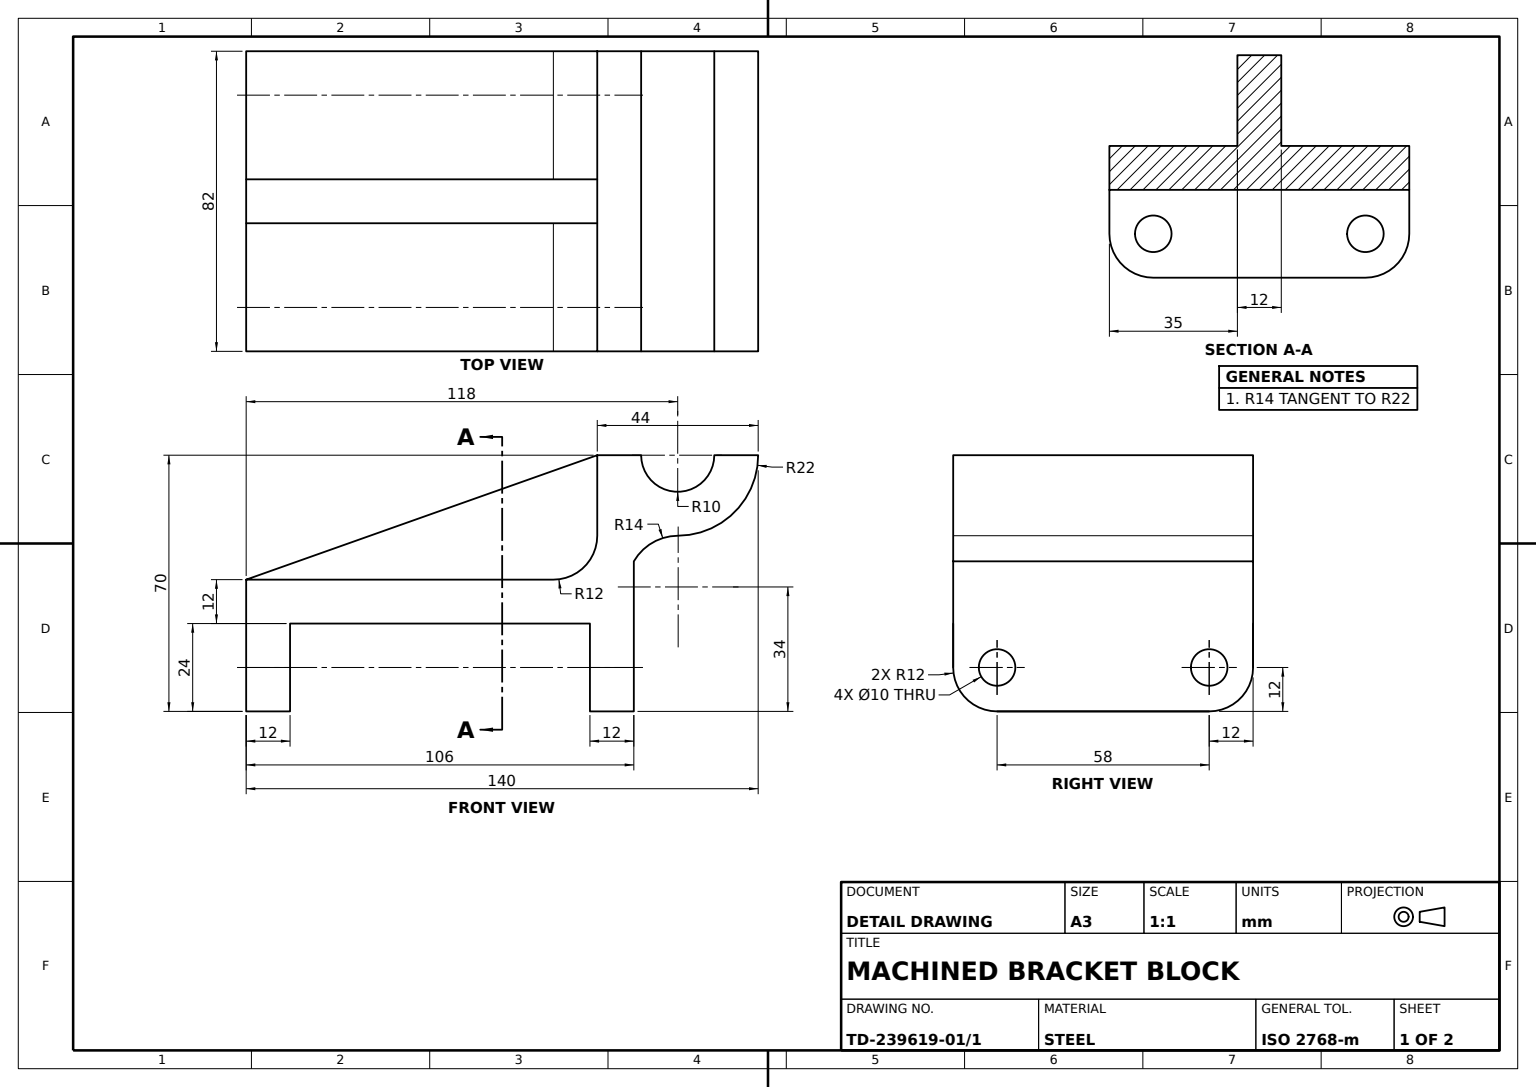
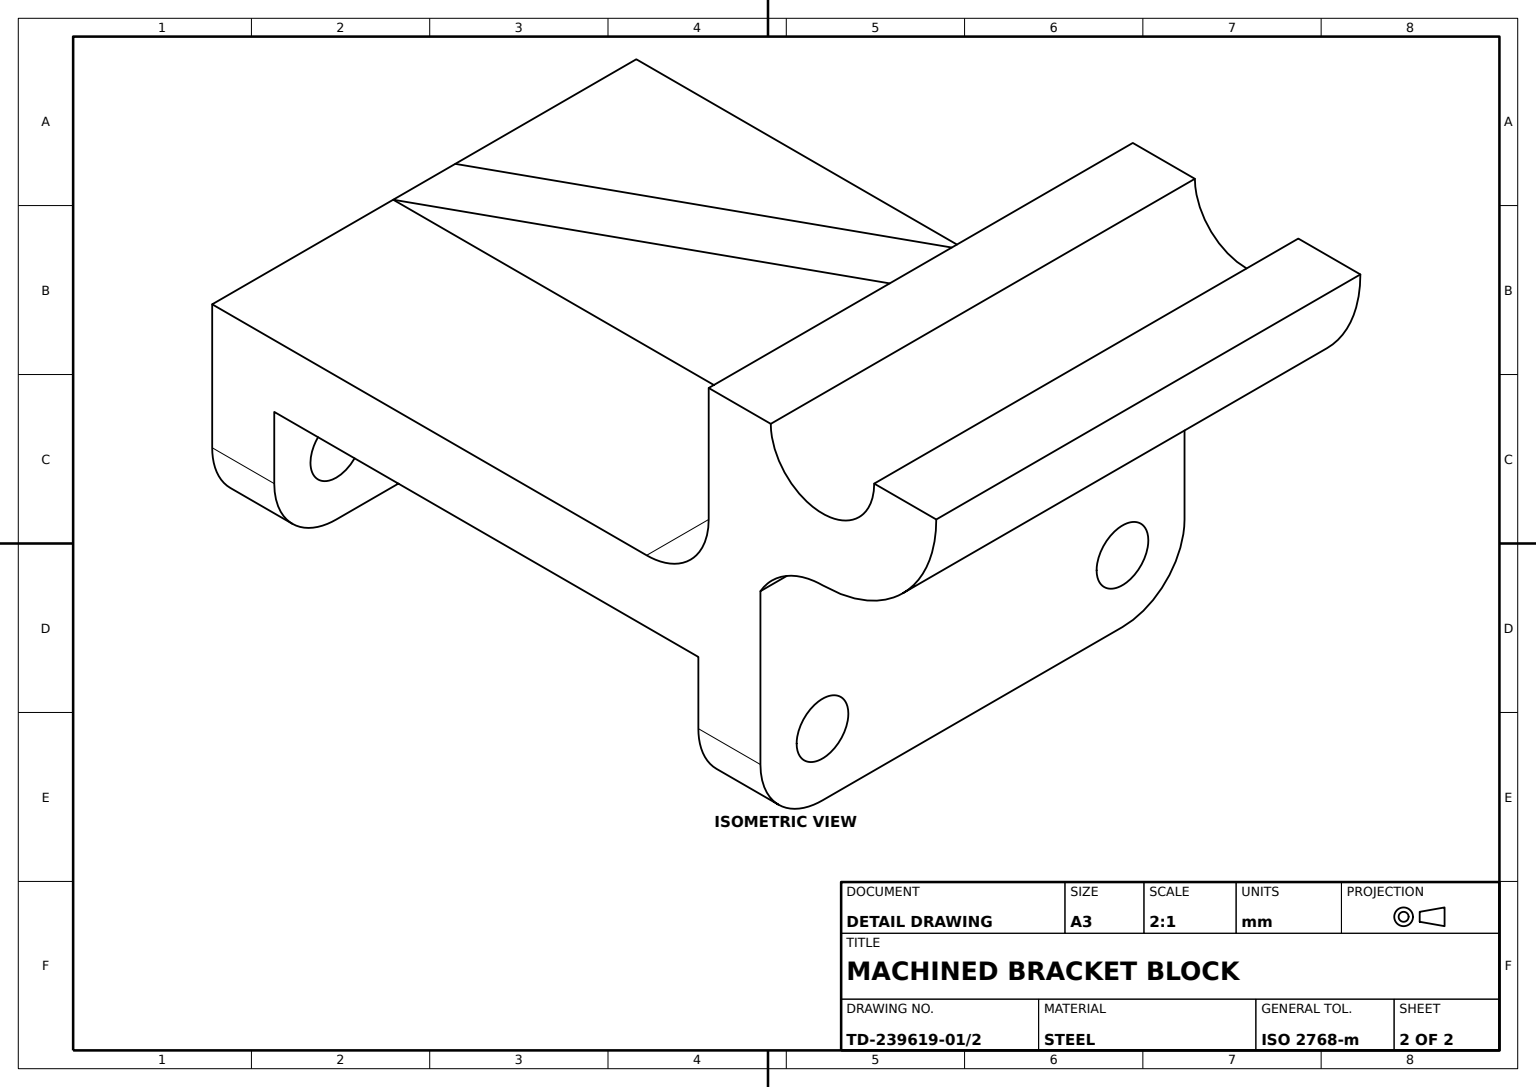
from build123d import *

# Parameters (mm, degrees)
BASE_PLATE_SKETCH_W       = 106
BASE_PLATE_SKETCH_H       = 82
BASE_PLATE_DEPTH          = 12
UPRIGHT_WALL_SKETCH_W     = 10
UPRIGHT_WALL_SKETCH_H     = 34
UPRIGHT_WALL_DEPTH        = 82
WALL_ROOT_FILLET_R12_R    = 12
MOUNTING_LUG_1_SKETCH_W   = 82
MOUNTING_LUG_1_SKETCH_H   = 24
MOUNTING_LUG_1_DEPTH      = 12
LUG_1_CORNER_FILLET_R12_R = 12
LUG_1_HOLE_SKETCH_R       = 5
LUG_1_MOUNTING_HOLE_DEPTH = 123.609135059
MOUNTING_LUG_2_SKETCH_W   = 82
MOUNTING_LUG_2_SKETCH_H   = 24
MOUNTING_LUG_2_DEPTH      = 12
LUG_2_CORNER_FILLET_R12_R = 12
LUG_START                 = -12
LUG_2_HOLE_SKETCH_R       = 5
LUG_2_MOUNTING_HOLE_DEPTH = 12
SIDE_SUPPORT_DEPTH        = 6
GROOVED_CLAMP_RAIL_DEPTH  = 82


with BuildPart() as part:
    # Base Plate Sketch → Base Plate (new body)
    with BuildSketch(Plane(origin=(0, 0, 0), x_dir=(1, 0, 0), z_dir=(0, 1, 0))):
        Rectangle(BASE_PLATE_SKETCH_W, BASE_PLATE_SKETCH_H)
    extrude(amount=BASE_PLATE_DEPTH)

    # Upright Wall Sketch → Upright Wall (add)
    with BuildSketch(Plane.XY.offset(41)):
        with Locations((48, 29)):
            Rectangle(UPRIGHT_WALL_SKETCH_W, UPRIGHT_WALL_SKETCH_H)
    extrude(amount=-UPRIGHT_WALL_DEPTH)

    # Wall Root Fillet R12
    wall_root_fillet_r12_edges = [part.edges().sort_by_distance(p)[0] for p in [
        (43, 12, 0),
    ]]
    fillet(wall_root_fillet_r12_edges, radius=WALL_ROOT_FILLET_R12_R)

    # Mounting Lug 1 Sketch → Mounting Lug 1 (add)
    with BuildSketch(Plane.ZY.offset(53)):
        with Locations((0, -12)):
            Rectangle(MOUNTING_LUG_1_SKETCH_W, MOUNTING_LUG_1_SKETCH_H)
    extrude(amount=-MOUNTING_LUG_1_DEPTH)

    # Lug 1 Corner Fillet R12
    lug_1_corner_fillet_r12_edges = [part.edges().sort_by_distance(p)[0] for p in [
        (-47, -24, -41),
        (-47, -24, 41),
    ]]
    fillet(lug_1_corner_fillet_r12_edges, radius=LUG_1_CORNER_FILLET_R12_R)

    # Lug 1 Hole Sketch → Lug 1 Mounting Hole (cut, through all)
    with BuildSketch(Plane.ZY.offset(53)):
        with Locations((-29, -12)):
            Circle(LUG_1_HOLE_SKETCH_R)
        with Locations((29, -12)):
            Circle(LUG_1_HOLE_SKETCH_R)
    extrude(amount=-LUG_1_MOUNTING_HOLE_DEPTH, mode=Mode.SUBTRACT)

    # Mounting Lug 2 Sketch → Mounting Lug 2 (add)
    with BuildSketch(Plane(origin=(53, 0, 0), x_dir=(0, 0, -1), z_dir=(1, 0, 0))):
        with Locations((0, -12)):
            Rectangle(MOUNTING_LUG_2_SKETCH_W, MOUNTING_LUG_2_SKETCH_H)
    extrude(amount=-MOUNTING_LUG_2_DEPTH)

    # Lug 2 Corner Fillet R12
    lug_2_corner_fillet_r12_edges = [part.edges().sort_by_distance(p)[0] for p in [
        (47, -24, 41),
        (47, -24, -41),
    ]]
    fillet(lug_2_corner_fillet_r12_edges, radius=LUG_2_CORNER_FILLET_R12_R)

    # Lug 2 Hole Sketch → Lug 2 Mounting Hole (cut)
    with BuildSketch(Plane(origin=(53, 0, 0), x_dir=(0, 0, -1), z_dir=(1, 0, 0)).offset(LUG_START)):
        with Locations(Location((-29, -12, 0), (0, 0, 180))):
            Circle(LUG_2_HOLE_SKETCH_R)
        with Locations(Location((29, -12, 0), (0, 0, 180))):
            Circle(LUG_2_HOLE_SKETCH_R)
    extrude(amount=LUG_2_MOUNTING_HOLE_DEPTH, mode=Mode.SUBTRACT)

    # Side Support Sketch → Side Support (add, symmetric)
    with BuildSketch(Plane.XY):
        with BuildLine():
            Line((-53, 12), (43, 46))
            Line((43, 46), (43, 24))
            ThreePointArc((43, 24), (39.485281374, 15.514718626), (31, 12))
            Line((31, 12), (-53, 12))
        make_face()
    extrude(amount=SIDE_SUPPORT_DEPTH, both=True)

    # Clamp Rail Profile Sketch → Grooved Clamp Rail (add)
    with BuildSketch(Plane.XY.offset(41)):
        with BuildLine():
            Line((53, 46), (55, 46))
            ThreePointArc((55, 46), (65, 36), (75, 46))
            Line((75, 46), (87, 46))
            ThreePointArc((87, 46), (80.583221155, 30.470569282), (65.076071052, 24.000131519))
            ThreePointArc((65.076071052, 24.000131519), (58.103421188, 22.112388202), (53, 17))
            Line((53, 17), (53, 46))
        make_face()
    extrude(amount=-GROOVED_CLAMP_RAIL_DEPTH)


solid = part.part
